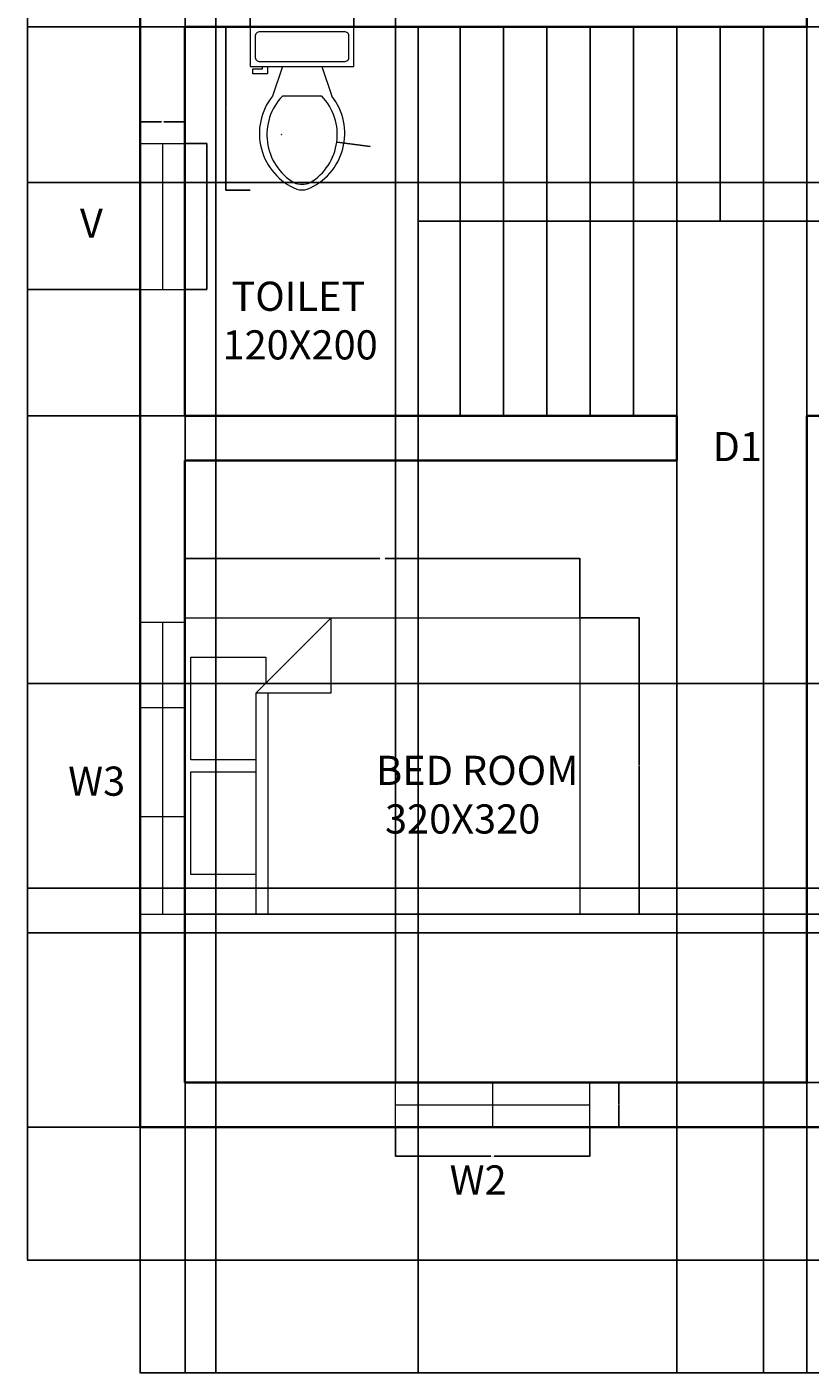
# Model space of a CAD drawing. Units: centimetres. Extents: x 575 to 1481, y 1225 to 2490.
# Tile 1 of 3: x 575 to 978, y 1225 to 1918. Entities that reach past the tile are written whole.
import ezdxf

# ---------------------------------------------------------------- set-up
doc = ezdxf.new("R2010")
doc.units = ezdxf.units.CM
for name, color, linetype, lineweight in [('A-ANNO-DIMS', 2, 'Continuous', 18), ('A-ANNO-TEXT', 3, 'Continuous', 18), ('A-AREA-IDEN', 7, 'Continuous', 18), ('A-FLOR-FIXT', 9, 'Continuous', 18), ('A-FLOR-STRS', 7, 'Continuous', 25), ('A-FURN', 8, 'Continuous', 18), ('A-GLAZ', 4, 'Continuous', 18), ('A-WALL', 7, 'Continuous', 35)]:
    doc.layers.add(name, color=color, linetype=linetype, lineweight=lineweight)
doc.styles.get("Standard").update_dxf_attribs({"font": 'arial.ttf'})
doc.dimstyles.get("Standard").update_dxf_attribs({"dimtxt": 0.18, "dimasz": 0.18, "dimexe": 0.18, "dimexo": 0.0625, "dimgap": 0.09, "dimtad": 0, "dimtih": 1, "dimtoh": 1, "dimdec": 4, "dimzin": 0, "dimdsep": 46, "dimtxsty": 'Standard', "dimcen": 0.09, "dimadec": 0, "dimazin": 0, "dimtfac": 1, "dimtdec": 4, "dimtofl": 0, "dimtmove": 0, "dimatfit": 3, "dimfxl": 1, "dimtolj": 1, "dimtzin": 0, "dimarcsym": 0})

# ---------------------------------------------------------------- blocks, each defined once
blk = doc.blocks.new('Toilet - top')
for p, q in [((9.5, -6), (9.5, -2)), ((-8, -8.5), (-8, -8)), ((-7, -8), (-7, -9.5)), ((-4, -8), (-6, -14)), ((4, -8), (6, -14)), ((-10, -8.5), (-8, -8.5)), ((-10, -9.5), (-10, -8.5)), ((-7, -9.5), (-10, -9.5)), ((4, -14), (-4, -14))]:
    blk.add_line(p, q)
blk.add_lwpolyline([(10.5, -8), (10.5, 0), (-10.5, 0), (-10.5, -8)], close=True)
for points in [[(-9.5, -2), (-9.5, -6)], [(8.5, -1), (-8.5, -1)], [(-8.5, -7), (8.5, -7)]]:
    blk.add_lwpolyline(points)
for centre, radius, start, end in [((-8.62, -1.88), 0.884, 81.8699, 188.1301), ((8.62, -1.88), 0.884, 351.8699, 98.1301), ((-8.62, -6.12), 0.884, 171.8699, 278.1301), ((8.62, -6.12), 0.884, 261.8699, 8.1301), ((3.52, -21.58), 12.17, 141.4691, 247.9714), ((4.2, -21.82), 11.33, 136.3677, 238.9468), ((-3.52, -21.58), 12.17, 292.0284, 38.5307), ((-4.2, -21.82), 11.33, 301.053, 43.6321), ((0, -27.88), 4, 245.7318, 294.2682), ((0, -29), 4, 254.8605, 285.1395)]:
    blk.add_arc(centre, radius, start, end)
blk = doc.blocks.new('Bed - Queen')
for p, q in [((0, -80.00003), (0, 0)), ((0, 0), (59.99999, 0)), ((59.99999, 0), (59.99999, -80.00003)), ((7.99999, -1.2), (28.79998, -1.2)), ((7.99999, -14.4), (7.99999, -1.2)), ((28.79998, -1.2), (28.79998, -14.4)), ((31.19999, -1.2), (51.99999, -1.2)), ((31.19999, -14.4), (31.19999, -1.2)), ((51.99999, -1.2), (51.99999, -16.4)), ((0, -14.4), (44.8, -14.4)), ((59.99999, -29.6), (44.8, -14.4)), ((44.8, -14.4), (44.8, -29.6)), ((44.8, -16.8), (0, -16.8)), ((51.99999, -16.4), (46.79936, -16.4)), ((44.8, -29.6), (59.99999, -29.6)), ((59.99999, -80.00003), (0, -80.00003))]:
    blk.add_line(p, q)
blk = doc.blocks.new('WIN-W2-100CM')
for p, q in [((0, 0), (0, 23)), ((50, 23), (50, 0)), ((100, 0), (100, 23)), ((0, 11.5), (100, 11.5))]:
    blk.add_line(p, q)
blk = doc.blocks.new('WIN-W3-150CM')
for p, q in [((11.5, 150), (11.5, 0)), ((0, 106.3), (23, 106.3)), ((0, 50.18), (23, 50.18))]:
    blk.add_line(p, q)
blk.add_lwpolyline([(23, 0), (23, 150), (0, 150), (0, 0)], close=True)
blk = doc.blocks.new('VENT-75CM')
for p, q in [((0, 23), (0, 0)), ((75, 23), (75, 0)), ((75, 11.5), (0, 11.5))]:
    blk.add_line(p, q)
blk = doc.blocks.new('*D10')
at = {"layer": 'A-ANNO-DIMS', "color": 0, "lineweight": -2, "transparency": 16777216}
for p, q in [((764.7, 1351.5), (764.7, 1336.39)), ((864.7, 1351.5), (864.7, 1336.39)), ((764.88, 1336.57), (813.87, 1336.57)), ((864.52, 1336.57), (815.53, 1336.57))]:
    blk.add_line(p, q, dxfattribs=at)
at = {"layer": 'A-ANNO-DIMS', "color": 0, "transparency": 16777216}
for points in [[(764.88, 1336.6), (764.88, 1336.54), (764.7, 1336.57)], [(864.52, 1336.6), (864.52, 1336.54), (864.7, 1336.57)]]:
    blk.add_solid(points, dxfattribs=at)
at = {"layer": 'Defpoints', "color": 0, "transparency": 16777216}
for p in [(764.7, 1351.57), (864.7, 1351.57), (864.7, 1336.57)]:
    blk.add_point(p, dxfattribs=at)
at = {"layer": 'A-ANNO-DIMS', "color": 0, "transparency": 16777216, "insert": (814.7, 1336.57), "char_height": 0.18, "attachment_point": 5}
blk.add_mtext('\\A1;W2 100 TYP.', dxfattribs=at)
blk = doc.blocks.new('*D11')
at = {"layer": 'A-ANNO-DIMS', "color": 0, "lineweight": -2, "transparency": 16777216}
for p, q in [((864.76, 1374.57), (879.88, 1374.57)), ((879.7, 1374.39), (879.7, 1363.25)), ((879.7, 1351.75), (879.7, 1362.88)), ((864.76, 1351.57), (879.88, 1351.57))]:
    blk.add_line(p, q, dxfattribs=at)
at = {"layer": 'A-ANNO-DIMS', "color": 0, "transparency": 16777216}
for points in [[(879.67, 1374.39), (879.73, 1374.39), (879.7, 1374.57)], [(879.67, 1351.75), (879.73, 1351.75), (879.7, 1351.57)]]:
    blk.add_solid(points, dxfattribs=at)
at = {"layer": 'Defpoints', "color": 0, "transparency": 16777216}
for p in [(864.7, 1374.57), (879.7, 1374.57), (864.7, 1351.57)]:
    blk.add_point(p, dxfattribs=at)
at = {"layer": 'A-ANNO-DIMS', "color": 0, "transparency": 16777216, "insert": (879.7, 1363.07), "char_height": 0.18, "attachment_point": 5}
blk.add_mtext('\\A1;23 TYP.', dxfattribs=at)
blk = doc.blocks.new('*D14')
at = {"layer": 'A-ANNO-DIMS', "color": 0, "lineweight": -2, "transparency": 16777216}
for p, q in [((656.52, 1857.57), (667.89, 1857.57)), ((667.71, 1857.39), (667.71, 1820.25)), ((667.71, 1782.75), (667.71, 1819.88)), ((656.52, 1782.57), (667.89, 1782.57))]:
    blk.add_line(p, q, dxfattribs=at)
at = {"layer": 'A-ANNO-DIMS', "color": 0, "transparency": 16777216}
for points in [[(667.68, 1857.39), (667.74, 1857.39), (667.71, 1857.57)], [(667.68, 1782.75), (667.74, 1782.75), (667.71, 1782.57)]]:
    blk.add_solid(points, dxfattribs=at)
at = {"layer": 'Defpoints', "color": 0, "transparency": 16777216}
for p in [(656.46, 1857.57), (667.71, 1857.57), (656.46, 1782.57)]:
    blk.add_point(p, dxfattribs=at)
at = {"layer": 'A-ANNO-DIMS', "color": 0, "transparency": 16777216, "insert": (667.71, 1820.07), "char_height": 0.18, "attachment_point": 5}
blk.add_mtext('\\A1;VENT 75 TYP.', dxfattribs=at)
blk = doc.blocks.new('*D15')
at = {"layer": 'A-ANNO-DIMS', "color": 0, "lineweight": -2, "transparency": 16777216}
for p, q in [((633.46, 1857.63), (633.46, 1869)), ((633.64, 1868.82), (644.43, 1868.82)), ((656.28, 1868.82), (645.49, 1868.82)), ((656.46, 1857.63), (656.46, 1869))]:
    blk.add_line(p, q, dxfattribs=at)
at = {"layer": 'A-ANNO-DIMS', "color": 0, "transparency": 16777216}
for points in [[(633.64, 1868.85), (633.64, 1868.79), (633.46, 1868.82)], [(656.28, 1868.85), (656.28, 1868.79), (656.46, 1868.82)]]:
    blk.add_solid(points, dxfattribs=at)
at = {"layer": 'Defpoints', "color": 0, "transparency": 16777216}
for p in [(633.46, 1868.82), (633.46, 1857.57), (656.46, 1857.57)]:
    blk.add_point(p, dxfattribs=at)
at = {"layer": 'A-ANNO-DIMS', "color": 0, "transparency": 16777216, "insert": (644.96, 1868.82), "char_height": 0.18, "attachment_point": 5}
blk.add_mtext('\\A1;23 TYP.', dxfattribs=at)
blk = doc.blocks.new('*D18')
at = {"layer": 'A-ANNO-DIMS', "color": 0, "lineweight": -2, "transparency": 16777216}
for p, q in [((656.46, 1613.66), (656.46, 1644.26)), ((656.64, 1644.08), (756.68, 1644.08)), ((859.48, 1644.08), (759.43, 1644.08)), ((859.66, 1613.66), (859.66, 1644.26))]:
    blk.add_line(p, q, dxfattribs=at)
at = {"layer": 'A-ANNO-DIMS', "color": 0, "transparency": 16777216}
for points in [[(656.64, 1644.11), (656.64, 1644.05), (656.46, 1644.08)], [(859.48, 1644.11), (859.48, 1644.05), (859.66, 1644.08)]]:
    blk.add_solid(points, dxfattribs=at)
at = {"layer": 'Defpoints', "color": 0, "transparency": 16777216}
for p in [(656.46, 1644.08), (656.46, 1613.6), (859.66, 1613.6)]:
    blk.add_point(p, dxfattribs=at)
at = {"layer": 'A-ANNO-DIMS', "color": 0, "transparency": 16777216, "insert": (758.06, 1644.08), "char_height": 0.18, "attachment_point": 5}
blk.add_mtext('\\A1;QUEEN BED 203 TYP.', dxfattribs=at)
blk = doc.blocks.new('*D19')
at = {"layer": 'A-ANNO-DIMS', "color": 0, "lineweight": -2, "transparency": 16777216}
for p, q in [((859.72, 1613.6), (890.32, 1613.6)), ((890.14, 1613.42), (890.14, 1537.58)), ((890.14, 1461.38), (890.14, 1537.22)), ((859.72, 1461.2), (890.32, 1461.2))]:
    blk.add_line(p, q, dxfattribs=at)
at = {"layer": 'A-ANNO-DIMS', "color": 0, "transparency": 16777216}
for points in [[(890.11, 1613.42), (890.17, 1613.42), (890.14, 1613.6)], [(890.11, 1461.38), (890.17, 1461.38), (890.14, 1461.2)]]:
    blk.add_solid(points, dxfattribs=at)
at = {"layer": 'Defpoints', "color": 0, "transparency": 16777216}
for p in [(859.66, 1613.6), (890.14, 1613.6), (859.66, 1461.2)]:
    blk.add_point(p, dxfattribs=at)
at = {"layer": 'A-ANNO-DIMS', "color": 0, "transparency": 16777216, "insert": (890.14, 1537.4), "char_height": 0.18, "attachment_point": 5}
blk.add_mtext('\\A1;152 TYP.', dxfattribs=at)
blk = doc.blocks.new('*D20')
at = {"layer": 'A-ANNO-DIMS', "color": 0, "lineweight": -2, "transparency": 16777216}
for p, q in [((689.97, 1917.57), (677.26, 1917.57)), ((677.44, 1917.39), (677.44, 1875.78)), ((677.44, 1833.81), (677.44, 1875.41)), ((689.97, 1833.63), (677.26, 1833.63))]:
    blk.add_line(p, q, dxfattribs=at)
at = {"layer": 'A-ANNO-DIMS', "color": 0, "transparency": 16777216}
for points in [[(677.41, 1917.39), (677.47, 1917.39), (677.44, 1917.57)], [(677.41, 1833.81), (677.47, 1833.81), (677.44, 1833.63)]]:
    blk.add_solid(points, dxfattribs=at)
at = {"layer": 'Defpoints', "color": 0, "transparency": 16777216}
for p in [(677.44, 1917.57), (690.03, 1917.57), (690.03, 1833.63)]:
    blk.add_point(p, dxfattribs=at)
at = {"layer": 'A-ANNO-DIMS', "color": 0, "transparency": 16777216, "insert": (677.44, 1875.6), "char_height": 0.18, "attachment_point": 5}
blk.add_mtext('\\A1;WC 84 TYP.', dxfattribs=at)
blk = doc.blocks.new('*D21')
at = {"layer": 'A-ANNO-DIMS', "color": 0, "lineweight": -2, "transparency": 16777216}
for p, q in [((690.03, 1917.63), (690.03, 1930.34)), ((690.21, 1930.16), (716.17, 1930.16)), ((743.19, 1930.16), (717.23, 1930.16)), ((743.37, 1917.63), (743.37, 1930.34))]:
    blk.add_line(p, q, dxfattribs=at)
at = {"layer": 'A-ANNO-DIMS', "color": 0, "transparency": 16777216}
for points in [[(690.21, 1930.19), (690.21, 1930.13), (690.03, 1930.16)], [(743.19, 1930.19), (743.19, 1930.13), (743.37, 1930.16)]]:
    blk.add_solid(points, dxfattribs=at)
at = {"layer": 'Defpoints', "color": 0, "transparency": 16777216}
for p in [(743.37, 1930.16), (690.03, 1917.57), (743.37, 1917.57)]:
    blk.add_point(p, dxfattribs=at)
at = {"layer": 'A-ANNO-DIMS', "color": 0, "transparency": 16777216, "insert": (716.7, 1930.16), "char_height": 0.18, "attachment_point": 5}
blk.add_mtext('\\A1;53 TYP.', dxfattribs=at)
blk = doc.blocks.new('*D28')
at = {"layer": 'A-ANNO-DIMS', "color": 0, "lineweight": -2, "transparency": 16777216}
for p, q in [((633.46, 1351.5), (633.46, 1225.06)), ((1422.46, 1351.5), (1422.46, 1225.06)), ((633.64, 1225.24), (1027.67, 1225.24)), ((1422.28, 1225.24), (1028.25, 1225.24))]:
    blk.add_line(p, q, dxfattribs=at)
at = {"layer": 'A-ANNO-DIMS', "color": 0, "transparency": 16777216}
for points in [[(633.64, 1225.27), (633.64, 1225.21), (633.46, 1225.24)], [(1422.28, 1225.27), (1422.28, 1225.21), (1422.46, 1225.24)]]:
    blk.add_solid(points, dxfattribs=at)
at = {"layer": 'Defpoints', "color": 0, "transparency": 16777216}
for p in [(633.46, 1351.57), (1422.46, 1351.57), (1422.46, 1225.24)]:
    blk.add_point(p, dxfattribs=at)
at = {"layer": 'A-ANNO-DIMS', "color": 0, "transparency": 16777216, "insert": (1027.96, 1225.24), "char_height": 0.18, "attachment_point": 5}
blk.add_mtext('\\A1;789', dxfattribs=at)
blk = doc.blocks.new('*D29')
at = {"layer": 'A-ANNO-DIMS', "color": 0, "lineweight": -2, "transparency": 16777216}
for p, q in [((959.64, 2431.95), (575.33, 2431.95)), ((575.51, 2431.77), (575.51, 1857.75)), ((575.51, 1283.37), (575.51, 1857.38)), ((999.39, 1283.19), (575.33, 1283.19))]:
    blk.add_line(p, q, dxfattribs=at)
at = {"layer": 'A-ANNO-DIMS', "color": 0, "transparency": 16777216}
for points in [[(575.48, 2431.77), (575.54, 2431.77), (575.51, 2431.95)], [(575.48, 1283.37), (575.54, 1283.37), (575.51, 1283.19)]]:
    blk.add_solid(points, dxfattribs=at)
at = {"layer": 'Defpoints', "color": 0, "transparency": 16777216}
for p in [(575.51, 2431.95), (959.71, 2431.95), (999.46, 1283.19)]:
    blk.add_point(p, dxfattribs=at)
at = {"layer": 'A-ANNO-DIMS', "color": 0, "transparency": 16777216, "insert": (575.51, 1857.57), "char_height": 0.18, "attachment_point": 5}
blk.add_mtext('\\A1;1148.8', dxfattribs=at)
blk = doc.blocks.new('*D30')
at = {"layer": 'A-ANNO-DIMS', "color": 0, "lineweight": -2, "transparency": 16777216}
for p, q in [((656.46, 1374.63), (656.46, 2490.08)), ((656.64, 2489.9), (710.12, 2489.9)), ((764.52, 2489.9), (711.03, 2489.9)), ((764.7, 1374.63), (764.7, 2490.08))]:
    blk.add_line(p, q, dxfattribs=at)
at = {"layer": 'A-ANNO-DIMS', "color": 0, "transparency": 16777216}
for points in [[(656.64, 2489.93), (656.64, 2489.87), (656.46, 2489.9)], [(764.52, 2489.93), (764.52, 2489.87), (764.7, 2489.9)]]:
    blk.add_solid(points, dxfattribs=at)
at = {"layer": 'Defpoints', "color": 0, "transparency": 16777216}
for p in [(764.7, 2489.9), (656.46, 1374.57), (764.7, 1374.57)]:
    blk.add_point(p, dxfattribs=at)
at = {"layer": 'A-ANNO-DIMS', "color": 0, "transparency": 16777216, "insert": (710.58, 2489.9), "char_height": 0.18, "attachment_point": 5}
blk.add_mtext('\\A1;108.24', dxfattribs=at)
blk = doc.blocks.new('*D32')
at = {"layer": 'A-ANNO-DIMS', "color": 0, "lineweight": -2, "transparency": 16777216}
for p, q in [((656.52, 1461.2), (1480.59, 1461.2)), ((1480.41, 1461.02), (1480.41, 1418.07)), ((1480.41, 1374.75), (1480.41, 1417.7)), ((656.52, 1374.57), (1480.59, 1374.57))]:
    blk.add_line(p, q, dxfattribs=at)
at = {"layer": 'A-ANNO-DIMS', "color": 0, "transparency": 16777216}
for points in [[(1480.38, 1461.02), (1480.44, 1461.02), (1480.41, 1461.2)], [(1480.38, 1374.75), (1480.44, 1374.75), (1480.41, 1374.57)]]:
    blk.add_solid(points, dxfattribs=at)
at = {"layer": 'Defpoints', "color": 0, "transparency": 16777216}
for p in [(656.46, 1461.2), (1480.41, 1461.2), (656.46, 1374.57)]:
    blk.add_point(p, dxfattribs=at)
at = {"layer": 'A-ANNO-DIMS', "color": 0, "transparency": 16777216, "insert": (1480.41, 1417.88), "char_height": 0.18, "attachment_point": 5}
blk.add_mtext('\\A1;86.63', dxfattribs=at)
blk = doc.blocks.new('*D33')
at = {"layer": 'A-ANNO-DIMS', "color": 0, "lineweight": -2, "transparency": 16777216}
for p, q in [((633.39, 1782.57), (575.33, 1782.57)), ((575.51, 1782.39), (575.51, 1750.25)), ((575.51, 1717.75), (575.51, 1749.88)), ((656.39, 1717.57), (575.33, 1717.57))]:
    blk.add_line(p, q, dxfattribs=at)
at = {"layer": 'A-ANNO-DIMS', "color": 0, "transparency": 16777216}
for points in [[(575.48, 1782.39), (575.54, 1782.39), (575.51, 1782.57)], [(575.48, 1717.75), (575.54, 1717.75), (575.51, 1717.57)]]:
    blk.add_solid(points, dxfattribs=at)
at = {"layer": 'Defpoints', "color": 0, "transparency": 16777216}
for p in [(633.46, 1782.57), (575.51, 1717.57), (656.46, 1717.57)]:
    blk.add_point(p, dxfattribs=at)
at = {"layer": 'A-ANNO-DIMS', "color": 0, "transparency": 16777216, "insert": (575.51, 1750.07), "char_height": 0.18, "attachment_point": 5}
blk.add_mtext('\\A1;65', dxfattribs=at)
blk = doc.blocks.new('*D37')
at = {"layer": 'A-ANNO-DIMS', "color": 0, "lineweight": -2, "transparency": 16777216}
for p, q in [((1076.46, 2363.5), (1076.46, 1225.06)), ((976.46, 2340.5), (976.46, 1225.06)), ((976.64, 1225.24), (1026.18, 1225.24)), ((1076.28, 1225.24), (1026.74, 1225.24))]:
    blk.add_line(p, q, dxfattribs=at)
at = {"layer": 'A-ANNO-DIMS', "color": 0, "transparency": 16777216}
for points in [[(976.64, 1225.27), (976.64, 1225.21), (976.46, 1225.24)], [(1076.28, 1225.27), (1076.28, 1225.21), (1076.46, 1225.24)]]:
    blk.add_solid(points, dxfattribs=at)
at = {"layer": 'Defpoints', "color": 0, "transparency": 16777216}
for p in [(1076.46, 2363.57), (976.46, 2340.57), (1076.46, 1225.24)]:
    blk.add_point(p, dxfattribs=at)
at = {"layer": 'A-ANNO-DIMS', "color": 0, "transparency": 16777216, "insert": (1026.46, 1225.24), "char_height": 0.18, "attachment_point": 5}
blk.add_mtext('\\A1;100', dxfattribs=at)
blk = doc.blocks.new('*D39')
at = {"layer": 'A-ANNO-DIMS', "color": 0, "lineweight": -2, "transparency": 16777216}
for p, q in [((1399.39, 1579.79), (575.33, 1579.79)), ((575.51, 1579.61), (575.51, 1527.36)), ((575.51, 1474.75), (575.51, 1527)), ((1399.39, 1474.57), (575.33, 1474.57))]:
    blk.add_line(p, q, dxfattribs=at)
at = {"layer": 'A-ANNO-DIMS', "color": 0, "transparency": 16777216}
for points in [[(575.48, 1579.61), (575.54, 1579.61), (575.51, 1579.79)], [(575.48, 1474.75), (575.54, 1474.75), (575.51, 1474.57)]]:
    blk.add_solid(points, dxfattribs=at)
at = {"layer": 'Defpoints', "color": 0, "transparency": 16777216}
for p in [(575.51, 1579.79), (1399.46, 1579.79), (1399.46, 1474.57)]:
    blk.add_point(p, dxfattribs=at)
at = {"layer": 'A-ANNO-DIMS', "color": 0, "transparency": 16777216, "insert": (575.51, 1527.18), "char_height": 0.18, "attachment_point": 5}
blk.add_mtext('\\A1;105.22', dxfattribs=at)
blk = doc.blocks.new('*D40')
at = {"layer": 'A-ANNO-DIMS', "color": 0, "lineweight": -2, "transparency": 16777216}
for p, q in [((1399.39, 1925.38), (575.33, 1925.38)), ((575.51, 1925.2), (575.51, 1881.66)), ((575.51, 1837.75), (575.51, 1881.29)), ((1399.39, 1837.57), (575.33, 1837.57))]:
    blk.add_line(p, q, dxfattribs=at)
at = {"layer": 'A-ANNO-DIMS', "color": 0, "transparency": 16777216}
for points in [[(575.48, 1925.2), (575.54, 1925.2), (575.51, 1925.38)], [(575.48, 1837.75), (575.54, 1837.75), (575.51, 1837.57)]]:
    blk.add_solid(points, dxfattribs=at)
at = {"layer": 'Defpoints', "color": 0, "transparency": 16777216}
for p in [(575.51, 1925.38), (1399.46, 1925.38), (1399.46, 1837.57)]:
    blk.add_point(p, dxfattribs=at)
at = {"layer": 'A-ANNO-DIMS', "color": 0, "transparency": 16777216, "insert": (575.51, 1881.47), "char_height": 0.18, "attachment_point": 5}
blk.add_mtext('\\A1;87.82', dxfattribs=at)
blk = doc.blocks.new('*D42')
at = {"layer": 'A-ANNO-DIMS', "color": 0, "lineweight": -2, "transparency": 16777216}
for p, q in [((976.52, 1917.57), (1480.59, 1917.57)), ((1480.41, 1917.39), (1480.41, 1867.75)), ((1480.41, 1817.75), (1480.41, 1867.38)), ((976.52, 1817.57), (1480.59, 1817.57))]:
    blk.add_line(p, q, dxfattribs=at)
at = {"layer": 'A-ANNO-DIMS', "color": 0, "transparency": 16777216}
for points in [[(1480.38, 1917.39), (1480.44, 1917.39), (1480.41, 1917.57)], [(1480.38, 1817.75), (1480.44, 1817.75), (1480.41, 1817.57)]]:
    blk.add_solid(points, dxfattribs=at)
at = {"layer": 'Defpoints', "color": 0, "transparency": 16777216}
for p in [(976.46, 1917.57), (1480.41, 1917.57), (976.46, 1817.57)]:
    blk.add_point(p, dxfattribs=at)
at = {"layer": 'A-ANNO-DIMS', "color": 0, "transparency": 16777216, "insert": (1480.41, 1867.57), "char_height": 0.18, "attachment_point": 5}
blk.add_mtext('\\A1;100', dxfattribs=at)
blk = doc.blocks.new('*D43')
at = {"layer": 'A-ANNO-DIMS', "color": 0, "lineweight": -2, "transparency": 16777216}
for p, q in [((954.16, 1817.5), (954.16, 1225.06)), ((976.46, 1817.5), (976.46, 1225.06)), ((954.34, 1225.24), (964.84, 1225.24)), ((976.28, 1225.24), (965.77, 1225.24))]:
    blk.add_line(p, q, dxfattribs=at)
at = {"layer": 'A-ANNO-DIMS', "color": 0, "transparency": 16777216}
for points in [[(954.34, 1225.27), (954.34, 1225.21), (954.16, 1225.24)], [(976.28, 1225.27), (976.28, 1225.21), (976.46, 1225.24)]]:
    blk.add_solid(points, dxfattribs=at)
at = {"layer": 'Defpoints', "color": 0, "transparency": 16777216}
for p in [(954.16, 1817.57), (976.46, 1817.57), (976.46, 1225.24)]:
    blk.add_point(p, dxfattribs=at)
at = {"layer": 'A-ANNO-DIMS', "color": 0, "transparency": 16777216, "insert": (965.31, 1225.24), "char_height": 0.18, "attachment_point": 5}
blk.add_mtext('\\A1;22.297', dxfattribs=at)
blk = doc.blocks.new('*D44')
at = {"layer": 'A-ANNO-DIMS', "color": 0, "lineweight": -2, "transparency": 16777216}
for p, q in [((976.46, 1717.5), (976.46, 1225.06)), ((909.57, 1694.5), (909.57, 1225.06)), ((909.75, 1225.24), (942.62, 1225.24)), ((976.28, 1225.24), (943.41, 1225.24))]:
    blk.add_line(p, q, dxfattribs=at)
at = {"layer": 'A-ANNO-DIMS', "color": 0, "transparency": 16777216}
for points in [[(909.75, 1225.27), (909.75, 1225.21), (909.57, 1225.24)], [(976.28, 1225.27), (976.28, 1225.21), (976.46, 1225.24)]]:
    blk.add_solid(points, dxfattribs=at)
at = {"layer": 'Defpoints', "color": 0, "transparency": 16777216}
for p in [(976.46, 1717.57), (909.57, 1694.57), (976.46, 1225.24)]:
    blk.add_point(p, dxfattribs=at)
at = {"layer": 'A-ANNO-DIMS', "color": 0, "transparency": 16777216, "insert": (943.01, 1225.24), "char_height": 0.18, "attachment_point": 5}
blk.add_mtext('\\A1;66.89', dxfattribs=at)
blk = doc.blocks.new('*D45')
at = {"layer": 'A-ANNO-DIMS', "color": 0, "lineweight": -2, "transparency": 16777216}
for p, q in [((776.46, 1717.5), (776.46, 1225.06)), ((909.57, 1717.5), (909.57, 1225.06)), ((776.64, 1225.24), (842.64, 1225.24)), ((909.39, 1225.24), (843.38, 1225.24))]:
    blk.add_line(p, q, dxfattribs=at)
at = {"layer": 'A-ANNO-DIMS', "color": 0, "transparency": 16777216}
for points in [[(776.64, 1225.27), (776.64, 1225.21), (776.46, 1225.24)], [(909.39, 1225.27), (909.39, 1225.21), (909.57, 1225.24)]]:
    blk.add_solid(points, dxfattribs=at)
at = {"layer": 'Defpoints', "color": 0, "transparency": 16777216}
for p in [(776.46, 1717.57), (909.57, 1717.57), (909.57, 1225.24)]:
    blk.add_point(p, dxfattribs=at)
at = {"layer": 'A-ANNO-DIMS', "color": 0, "transparency": 16777216, "insert": (843.01, 1225.24), "char_height": 0.18, "attachment_point": 5}
blk.add_mtext('\\A1;133.1', dxfattribs=at)
blk = doc.blocks.new('*D46')
at = {"layer": 'A-ANNO-DIMS', "color": 0, "lineweight": -2, "transparency": 16777216}
for p, q in [((1076.39, 1917.57), (575.33, 1917.57)), ((575.51, 1917.39), (575.51, 1877.75)), ((575.51, 1837.75), (575.51, 1877.38)), ((1076.39, 1837.57), (575.33, 1837.57))]:
    blk.add_line(p, q, dxfattribs=at)
at = {"layer": 'A-ANNO-DIMS', "color": 0, "transparency": 16777216}
for points in [[(575.48, 1917.39), (575.54, 1917.39), (575.51, 1917.57)], [(575.48, 1837.75), (575.54, 1837.75), (575.51, 1837.57)]]:
    blk.add_solid(points, dxfattribs=at)
at = {"layer": 'Defpoints', "color": 0, "transparency": 16777216}
for p in [(575.51, 1917.57), (1076.46, 1917.57), (1076.46, 1837.57)]:
    blk.add_point(p, dxfattribs=at)
at = {"layer": 'A-ANNO-DIMS', "color": 0, "transparency": 16777216, "insert": (575.51, 1877.57), "char_height": 0.18, "attachment_point": 5}
blk.add_mtext('\\A1;80', dxfattribs=at)
blk = doc.blocks.new('*D54')
at = {"layer": 'A-ANNO-DIMS', "color": 0, "lineweight": -2, "transparency": 16777216}
for p, q in [((656.46, 2119.61), (656.46, 1225.06)), ((672.3, 2090.01), (672.3, 1225.06)), ((656.64, 1225.24), (663.99, 1225.24)), ((672.12, 1225.24), (664.76, 1225.24))]:
    blk.add_line(p, q, dxfattribs=at)
at = {"layer": 'A-ANNO-DIMS', "color": 0, "transparency": 16777216}
for points in [[(656.64, 1225.27), (656.64, 1225.21), (656.46, 1225.24)], [(672.12, 1225.27), (672.12, 1225.21), (672.3, 1225.24)]]:
    blk.add_solid(points, dxfattribs=at)
at = {"layer": 'Defpoints', "color": 0, "transparency": 16777216}
for p in [(656.46, 2119.68), (672.3, 2090.08), (672.3, 1225.24)]:
    blk.add_point(p, dxfattribs=at)
at = {"layer": 'A-ANNO-DIMS', "color": 0, "transparency": 16777216, "insert": (664.38, 1225.24), "char_height": 0.18, "attachment_point": 5}
blk.add_mtext('\\A1;15.84', dxfattribs=at)
blk = doc.blocks.new('*D57')
at = {"layer": 'A-ANNO-DIMS', "color": 0, "lineweight": -2, "transparency": 16777216}
for p, q in [((1422.39, 1451.57), (575.33, 1451.57)), ((575.51, 1451.39), (575.51, 1401.75)), ((575.51, 1351.75), (575.51, 1401.38)), ((1422.39, 1351.57), (575.33, 1351.57))]:
    blk.add_line(p, q, dxfattribs=at)
at = {"layer": 'A-ANNO-DIMS', "color": 0, "transparency": 16777216}
for points in [[(575.48, 1451.39), (575.54, 1451.39), (575.51, 1451.57)], [(575.48, 1351.75), (575.54, 1351.75), (575.51, 1351.57)]]:
    blk.add_solid(points, dxfattribs=at)
at = {"layer": 'Defpoints', "color": 0, "transparency": 16777216}
for p in [(575.51, 1451.57), (1422.46, 1451.57), (1422.46, 1351.57)]:
    blk.add_point(p, dxfattribs=at)
at = {"layer": 'A-ANNO-DIMS', "color": 0, "transparency": 16777216, "insert": (575.51, 1401.57), "char_height": 0.18, "attachment_point": 5}
blk.add_mtext('\\A1;100', dxfattribs=at)
blk = doc.blocks.new('*D61')
at = {"layer": 'A-ANNO-DIMS', "color": 0, "lineweight": -2, "transparency": 16777216}
for p, q in [((705.94, 1862.15), (706.12, 1862.15)), ((706.03, 1862.06), (706.03, 1862.24)), ((751.66, 1856.01), (734.73, 1858.29))]:
    blk.add_line(p, q, dxfattribs=at)
at = {"layer": 'A-ANNO-DIMS', "color": 0, "transparency": 16777216}
blk.add_solid([(734.73, 1858.32), (734.73, 1858.26), (734.55, 1858.31)], dxfattribs=at)
at = {"layer": 'Defpoints', "color": 0, "transparency": 16777216}
for p in [(706.03, 1862.15), (734.55, 1858.31)]:
    blk.add_point(p, dxfattribs=at)
at = {"layer": 'A-ANNO-DIMS', "color": 0, "transparency": 16777216, "insert": (752.41, 1856.01), "char_height": 0.18, "attachment_point": 5}
blk.add_mtext('\\A1;4X R28.776', dxfattribs=at)

msp = doc.modelspace()

# ---------------------------------------------------------------- linework, layer by layer
at = {"layer": 'A-FLOR-STRS'}
for p, q in [((776.457, 1917.566), (776.457, 1817.566)), ((798.0787, 1917.566), (798.0787, 1817.566)), ((820.376, 1917.566), (820.376, 1817.566)), ((842.6733, 1917.566), (842.6733, 1817.566)), ((864.9706, 1917.566), (864.9706, 1817.566)), ((887.2678, 1917.566), (887.2678, 1817.566)), ((909.5651, 1917.566), (909.5651, 1817.566)), ((931.8624, 1917.566), (931.8624, 1817.566)), ((954.1597, 1917.566), (954.1597, 1817.566)), ((976.457, 1917.566), (976.457, 1817.566)), ((976.457, 1817.566), (776.457, 1817.566)), ((776.457, 1817.566), (776.457, 1717.566)), ((798.0787, 1817.566), (798.0787, 1717.566)), ((820.376, 1817.566), (820.376, 1717.566)), ((842.6733, 1817.566), (842.6733, 1717.566)), ((864.9706, 1817.566), (864.9706, 1717.566)), ((887.2678, 1817.566), (887.2678, 1717.566)), ((909.5651, 1817.566), (909.5651, 1717.566))]:
    msp.add_line(p, q, dxfattribs=at)
at = {"layer": 'A-WALL'}
for p, q in [((633.457, 2363.566), (633.457, 1351.566)), ((976.457, 1940.566), (976.457, 1917.566)), ((656.457, 1917.566), (976.457, 1917.566)), ((656.457, 1917.566), (656.457, 1717.566)), ((656.457, 1717.566), (909.5651, 1717.566)), ((909.5651, 1717.566), (909.5651, 1694.566)), ((976.457, 1717.566), (976.457, 1374.566)), ((976.457, 1717.566), (999.457, 1717.566)), ((656.457, 1694.566), (909.5651, 1694.566)), ((656.457, 1694.566), (656.457, 1374.566)), ((656.457, 1374.566), (976.457, 1374.566)), ((633.457, 1351.566), (999.457, 1351.566))]:
    msp.add_line(p, q, dxfattribs=at)

# ---------------------------------------------------------------- block references
at = {"layer": 'A-FLOR-FIXT', "xscale": 2.54, "yscale": 2.54, "zscale": 2.54}
msp.add_blockref('Toilet - top', (716.6995, 1917.566), dxfattribs=at)
at = {"layer": 'A-FURN', "xscale": 2.54, "yscale": 2.54, "zscale": 2.54, "rotation": 90}
msp.add_blockref('Bed - Queen', (656.457, 1461.2007), dxfattribs=at)
at = {"layer": 'A-GLAZ', "rotation": 89.99999999999936}
msp.add_blockref('VENT-75CM', (656.457, 1782.5657), dxfattribs=at)
at = {"layer": 'A-GLAZ'}
for name, p in [('WIN-W3-150CM', (633.457, 1461.2004)), ('WIN-W2-100CM', (764.7005, 1351.566))]:
    msp.add_blockref(name, p, dxfattribs=at)

# ---------------------------------------------------------------- texts
at = {"layer": 'A-ANNO-TEXT', "char_height": 15, "attachment_point": 1}
for s, insert in [('V', (602.4145, 1824.0696)), ('D1', (927.8694, 1709.1766)), ('W3', (596.3484, 1537.0502)), ('W2', (792.6132, 1331.9036))]:
    msp.add_mtext_dynamic_manual_height_columns(s, width=230.89075, gutter_width=12.5, heights=[0], dxfattribs=dict(at, insert=insert))
at = {"layer": 'A-AREA-IDEN', "char_height": 15, "attachment_point": 1}
for s, insert in [(' TOILET\\P120X200', (675.7633, 1786.5052)), ('BED ROOM \\P 320X320', (754.7732, 1542.6175))]:
    msp.add_mtext_dynamic_manual_height_columns(s, width=230.89075, gutter_width=12.5, heights=[0], dxfattribs=dict(at, insert=insert))

# ---------------------------------------------------------------- dimensions: what is measured, and where the dimension line sits
at = {"layer": 'A-ANNO-DIMS'}
for base, p1, p2, override, picture, middle in [((764.7001, 2489.8956), (656.457, 1374.566), (764.7001, 1374.566), {"dimdec": 2, "dimlfac": 1, "dimrnd": 0, "dimzin": 0, "dimdsep": 46, "dimlunit": 2}, '*D30', (710.5785, 2489.8956)), ((1076.457, 1225.2364), (976.457, 2340.566), (1076.457, 2363.566), {"dimdec": 0, "dimlfac": 1, "dimrnd": 0, "dimzin": 0, "dimdsep": 46, "dimlunit": 2}, '*D37', (1026.457, 1225.2364)), ((672.2969, 1225.2364), (656.457, 2119.6752), (672.2969, 2090.0753), {"dimdec": 2, "dimlfac": 1, "dimrnd": 0, "dimzin": 0, "dimdsep": 46, "dimlunit": 2}, '*D54', (664.3769, 1225.2364)), ((976.457, 1225.2364), (954.1597, 1817.566), (976.457, 1817.566), {"dimdec": 3, "dimlfac": 1, "dimrnd": 0, "dimzin": 0, "dimdsep": 46, "dimlunit": 2}, '*D43', (965.3083, 1225.2364)), ((909.5651, 1225.2364), (776.457, 1717.566), (909.5651, 1717.566), {"dimdec": 1, "dimlfac": 1, "dimrnd": 0, "dimzin": 0, "dimdsep": 46, "dimlunit": 2}, '*D45', (843.011, 1225.2364)), ((976.457, 1225.2364), (909.5651, 1694.566), (976.457, 1717.566), {"dimdec": 2, "dimlfac": 1, "dimrnd": 0, "dimzin": 0, "dimdsep": 46, "dimlunit": 2}, '*D44', (943.011, 1225.2364)), ((1422.457, 1225.2364), (633.457, 1351.566), (1422.457, 1351.566), {"dimdec": 0, "dimlfac": 1, "dimrnd": 0, "dimzin": 0, "dimdsep": 46, "dimlunit": 2}, '*D28', (1027.957, 1225.2364))]:
    dim = msp.add_linear_dim(base=base, p1=p1, p2=p2, dimstyle='Standard', override=override, dxfattribs=at)
    dim.commit()
    dim.dimension.update_dxf_attribs({"geometry": picture, "text_midpoint": middle})
for base, p1, p2, override, picture, middle in [((575.507, 2431.9456), (999.457, 1283.1864), (959.7054, 2431.9456), {"dimdec": 1, "dimlfac": 1, "dimrnd": 0, "dimzin": 0, "dimdsep": 46, "dimlunit": 2}, '*D29', (575.507, 1857.566)), ((575.507, 1925.3838), (1399.457, 1837.566), (1399.457, 1925.3838), {"dimdec": 2, "dimlfac": 1, "dimrnd": 0, "dimzin": 0, "dimdsep": 46, "dimlunit": 2}, '*D40', (575.507, 1881.4749)), ((575.507, 1917.566), (1076.457, 1837.566), (1076.457, 1917.566), {"dimdec": 0, "dimlfac": 1, "dimrnd": 0, "dimzin": 0, "dimdsep": 46, "dimlunit": 2}, '*D46', (575.507, 1877.566)), ((1480.407, 1917.566), (976.457, 1817.566), (976.457, 1917.566), {"dimdec": 0, "dimlfac": 1, "dimrnd": 0, "dimzin": 0, "dimdsep": 46, "dimlunit": 2}, '*D42', (1480.407, 1867.566)), ((575.507, 1717.566), (633.457, 1782.566), (656.457, 1717.566), {"dimdec": 0, "dimlfac": 1, "dimrnd": 0, "dimzin": 0, "dimdsep": 46, "dimlunit": 2}, '*D33', (575.507, 1750.066)), ((575.507, 1579.7906), (1399.457, 1474.566), (1399.457, 1579.7906), {"dimdec": 2, "dimlfac": 1, "dimrnd": 0, "dimzin": 0, "dimdsep": 46, "dimlunit": 2}, '*D39', (575.507, 1527.1783)), ((1480.407, 1461.2007), (656.457, 1374.566), (656.457, 1461.2007), {"dimdec": 2, "dimlfac": 1, "dimrnd": 0, "dimzin": 0, "dimdsep": 46, "dimlunit": 2}, '*D32', (1480.407, 1417.8834)), ((575.507, 1451.566), (1422.457, 1351.566), (1422.457, 1451.566), {"dimdec": 0, "dimlfac": 1, "dimrnd": 0, "dimzin": 0, "dimdsep": 46, "dimlunit": 2}, '*D57', (575.507, 1401.566))]:
    dim = msp.add_linear_dim(base=base, p1=p1, p2=p2, angle=90, dimstyle='Standard', override=override, dxfattribs=at)
    dim.commit()
    dim.dimension.update_dxf_attribs({"geometry": picture, "text_midpoint": middle})
for base, p1, p2, text, picture, middle in [((743.3695, 1930.1567), (690.0295, 1917.566), (743.3695, 1917.566), '<> TYP.', '*D21', (716.6995, 1930.1567)), ((864.7001, 1336.566), (764.7001, 1351.566), (864.7001, 1351.566), 'W2 <> TYP.', '*D10', (814.7001, 1336.566))]:
    dim = msp.add_linear_dim(base=base, p1=p1, p2=p2, text=text, dimstyle='Standard', override={"dimdec": 0, "dimlfac": 1, "dimrnd": 0, "dimzin": 0, "dimdsep": 46, "dimlunit": 2}, dxfattribs=at)
    dim.commit()
    dim.dimension.update_dxf_attribs({"geometry": picture, "text_midpoint": middle})
for base, p1, p2, angle, text, picture, middle in [((677.4389, 1917.566), (690.0295, 1833.6286), (690.0295, 1917.566), 90, 'WC <> TYP.', '*D20', (677.4389, 1875.5973)), ((633.457, 1868.816), (656.457, 1857.566), (633.457, 1857.566), 180, '<> TYP.', '*D15', (644.957, 1868.816)), ((667.707, 1857.566), (656.457, 1782.566), (656.457, 1857.566), 90, 'VENT <> TYP.', '*D14', (667.707, 1820.066)), ((656.457, 1644.0807), (859.657, 1613.6007), (656.457, 1613.6007), 180, 'QUEEN BED <> TYP.', '*D18', (758.057, 1644.0807)), ((890.137, 1613.6007), (859.657, 1461.2007), (859.657, 1613.6007), 90, '<> TYP.', '*D19', (890.137, 1537.4007)), ((879.7001, 1374.566), (864.7001, 1351.566), (864.7001, 1374.566), 90, '<> TYP.', '*D11', (879.7001, 1363.066))]:
    dim = msp.add_linear_dim(base=base, p1=p1, p2=p2, angle=angle, text=text, dimstyle='Standard', override={"dimdec": 0, "dimlfac": 1, "dimrnd": 0, "dimzin": 0, "dimdsep": 46, "dimlunit": 2}, dxfattribs=at)
    dim.commit()
    dim.dimension.update_dxf_attribs({"geometry": picture, "text_midpoint": middle})
dim = msp.add_radius_dim(center=(706.0318, 1862.1499), mpoint=(734.5512, 1858.315), text='4X <>', dimstyle='Standard', override={"dimdec": 3, "dimlfac": 1, "dimrnd": 0, "dimzin": 0, "dimdsep": 46, "dimlunit": 2}, dxfattribs=at)
dim.commit()
dim.dimension.update_dxf_attribs({"geometry": '*D61', "text_midpoint": (751.6629, 1856.014), "dimtype": 164})

doc.saveas('drawing.dxf')
